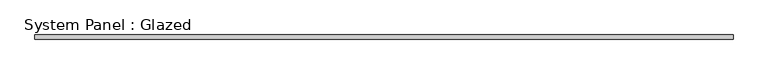
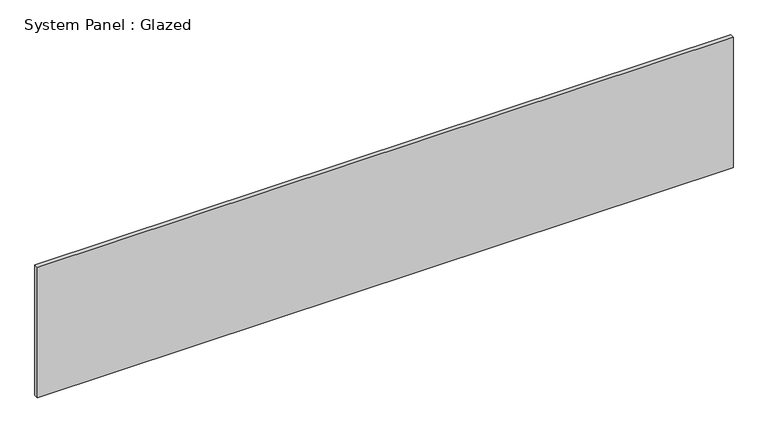
"""IFC4 building model written with IfcOpenShell, lengths in millimetres: plate geometry, System Panel : Glazed."""

from ifc_helpers import new_model, si_unit, origin, origin_with_axes, place, context, project, spatial, polyline, outline, extrude, source, transform, mapped, element, save


def system_panel_glazed_41d8189d(model_context):
    return source(origin(), model_context, "Body", "SweptSolid", [
        extrude(outline(polyline([(2146.3, 19.05), (-2146.3, 19.05), (-2146.3, 44.45), (2146.3, 44.45), (2146.3, 19.05)])), origin_with_axes(), (0.0, 0.0, 1.0), 850.9),
    ])


if __name__ == "__main__":
    model = new_model("IFC4")
    model_context = context("Model", 3, world=origin())
    ifc_project = project(units=[si_unit("LENGTHUNIT", "METRE", prefix="MILLI")], contexts=[model_context])
    site = spatial("IfcSite", under=ifc_project)
    building = spatial("IfcBuilding", under=site)
    placement = place(None, origin())
    system_panel_glazed_shape = system_panel_glazed_41d8189d(model_context)
    element("IfcPlate", 1, ObjectType="System Panel : Glazed", at=placement, inside=building, context=model_context, shape_type="MappedRepresentation", body=[
        mapped(system_panel_glazed_shape, transform((0.0, 0.0, 0.0), x_axis=(1.0, 0.0, 0.0), y_axis=(0.0, 1.0, 0.0), z_axis=(0.0, 0.0, 1.0))),
    ])
    save(model, "model.ifc")

# Revit data of these elements
# Type "System Panel : Glazed"
#   Construction Type Id = "GSP4R"
#   Analytic Construction = "1/8 in Pilkington single glazing"
#   Visual Light Transmittance = 0.9
#   Solar Heat Gain Coefficient = 0.86
#   Heat Transfer Coefficient (U) = 1.18115 BTU/(h·ft²·°F)
# Element 1 (IfcPlate, "System Panel : Glazed")
#   Materials on its faces: "Glass"
# Materials
#   "Glass": class "Glass", colour RGB 0 128 192, transparency 0.75, Description = "Soda Lime Glass", Cost = 0
